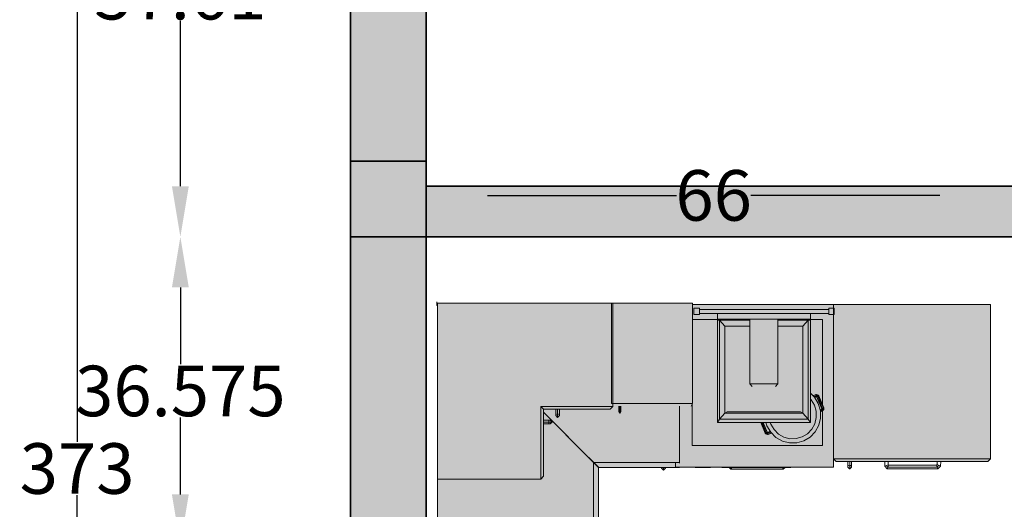
# Model space of a CAD drawing. Units: inches. Extents: x 1994 to 3075, y 3517 to 3950.
# Tile 50 of 58: x 2630 to 2747, y 3723 to 3781. Entities that reach past the tile are written whole.
import ezdxf

# ---------------------------------------------------------------- set-up
doc = ezdxf.new("R2010")
doc.units = ezdxf.units.IN
for name, color, linetype, lineweight in [('A-ANNO-DIMS', 2, 'Continuous', 18), ('A-COLS', 7, 'Continuous', 35), ('A-COLS-PATT', 6, 'Continuous', 13), ('A-FLOR-FIXT', 8, 'Continuous', 18), ('A-WALL', 7, 'Continuous', 35), ('A-WALL-PATT', 252, 'Continuous', 13)]:
    doc.layers.add(name, color=color, linetype=linetype, lineweight=lineweight)
doc.layers.add('hatch', color=254, linetype='Continuous')
doc.styles.get("Standard").update_dxf_attribs({"font": 'arial.ttf'})
doc.dimstyles.get("Standard").update_dxf_attribs({"dimtxt": 6, "dimasz": 6, "dimexe": 0.18, "dimexo": 0.0625, "dimgap": 0.09, "dimtad": 0, "dimtih": 1, "dimtoh": 1, "dimdec": 4, "dimzin": 0, "dimdsep": 46, "dimlunit": 4, "dimtxsty": 'Standard', "dimcen": 0.09, "dimse1": 1, "dimse2": 1, "dimadec": 0, "dimazin": 0, "dimtfac": 1, "dimtdec": 4, "dimtofl": 0, "dimtmove": 0, "dimatfit": 3, "dimfxl": 1, "dimtolj": 1, "dimtzin": 0, "dimarcsym": 0})

# ---------------------------------------------------------------- blocks, each defined once
blk = doc.blocks.new('kithen1')
at = {"layer": 'hatch'}
blk.add_hatch(color=256, dxfattribs=at).paths.add_polyline_path([(-2799.7, -8.3), (-2273.3, -8.3), (-2273.3, -1.7), (-2257.5, -1.7), (-2257.5, -1.1), (-1023.7, -1.1), (-1023.7, 0), (0, 0), (0, -0.3), (0.3, -0.3), (0.3, -1009.9), (-6.1, -1009.9), (-6.1, -2189.3), (-615.8, -2189.3), (-626.5, -2178.9), (-626.5, -1578.2), (-615.8, -1567.8), (-649.5, -1567.8), (-649.5, -1399.1), (-650.3, -1399.1), (-650.3, -1376.8), (-657.9, -1368.5), (-657.8, -1162.4), (-650.3, -1155.1), (-650.3, -1126.4), (-649.5, -1126.4), (-649.5, -1081.1), (-650.3, -1081.1), (-650.3, -1021.1), (-649.5, -1021.1), (-649.5, -959.1), (-651, -959.1), (-650.7, -903), (-653.5, -903), (-660.6, -895.5), (-660.5, -894.6), (-653.5, -887.1), (-651, -887.1), (-651, -638.7), (-651.2, -638.5), (-898.3, -638.5), (-898.3, -640.4), (-905.9, -647.4), (-906.8, -647.4), (-914.3, -640.4), (-914.3, -638.5), (-971.4, -638.5), (-971.4, -642.6), (-1016.2, -642.6), (-1016.2, -643.9), (-1023.8, -650.9), (-1024.7, -650.9), (-1032.2, -643.9), (-1032.2, -642.6), (-1179.7, -642.6), (-1188.8, -650.9), (-1395.6, -650.9), (-1403.7, -642.6), (-1813.5, -642.6), (-1822.6, -650.9), (-2029.4, -650.9), (-2037.5, -642.6), (-2257.5, -642.6), (-2257.5, -618.1), (-2261.3, -618.1), (-2271.7, -628.7), (-2458, -628.7), (-2727.7, -628.7), (-2727.7, -651.1), (-2735, -658.1), (-2735.9, -658), (-2743.2, -651.1), (-2743.2, -628.7), (-2789.4, -628.7), (-2799.7, -618.1)])
at = {"color": 0}
for p, q in [((0, 0), (-1023.7, 0)), ((-696.5, 0), (-696.5, -409.2)), ((-8.6, 1.9), (-10.5, 0)), ((-10.1, 0), (-8.2, 1.9)), ((-8.2, 1.9), (-8.3, 1.8)), ((-8.3, 1.9), (-8.3, 0)), ((5.4, 1.8), (-8.3, 1.8)), ((0, 0), (0, -694.7)), ((0, -0.3), (0, 0)), ((0.3, -0.3), (0, -0.3)), ((0.3, -671.1), (0.3, -0.3)), ((-696.5, -409.2), (-408.8, -409.2)), ((-685.5, -420.3), (-696.5, -409.2)), ((-419.9, -420.3), (-685.5, -420.3)), ((-432.1, -420.3), (-630.9, -618.1)), ((-630.6, -618.4), (-431.9, -420.3)), ((-614.8, -602.2), (-432.2, -420.3)), ((-431.9, -420.3), (-614.5, -602.5)), ((-432, -420.3), (-607.9, -595.8)), ((-432.1, -420.3), (-607.9, -595.4)), ((-478.5, -420.3), (-478.5, -439.9)), ((-470.7, -443), (-470.7, -420.3)), ((-462.9, -420.3), (-462.9, -439.9)), ((-408.8, -409.2), (-419.9, -420.3)), ((-419.9, -683.7), (-419.9, -420.3)), ((-408.8, -409.2), (-408.8, -694.7)), ((-478.5, -439.9), (-470.7, -443)), ((-478.5, -439.9), (-478.5, -446.8)), ((-478.5, -446.8), (-470.7, -454.1)), ((-462.9, -439.9), (-470.7, -443)), ((-470.7, -443), (-470.7, -454.1)), ((-470.7, -454.1), (-462.9, -446.8)), ((-462.9, -446.8), (-462.9, -439.9)), ((-444.9, -468.4), (-452.2, -476.2)), ((-452.2, -476.2), (-441.1, -476.2)), ((-452.2, -476.2), (-444.9, -484)), ((-419.9, -468.4), (-444.9, -468.4)), ((-444.9, -484), (-438, -484)), ((-441.1, -476.2), (-438, -468.4)), ((-419.9, -476.2), (-441.1, -476.2)), ((-441.1, -476.2), (-438, -484)), ((-438, -484), (-419.9, -484)), ((-540.1, -527.9), (-540.1, -528.1)), ((-597, -584.5), (-597, -584.9)), ((-630.9, -618.1), (-971.4, -618.1)), ((-611.6, -599.1), (-651.2, -638.5)), ((-611.6, -599.4), (-651, -638.7)), ((-642.6, -629.8), (-630.9, -618.1)), ((-630.6, -618.4), (-642.3, -630.1)), ((-630.9, -618.1), (-614.8, -602.2)), ((-614.5, -602.5), (-630.6, -618.4)), ((-630.6, -959.1), (-630.6, -618.4)), ((-620.1, -607.7), (-609.4, -597.1)), ((-619.9, -607.6), (-620.1, -607.6)), ((-620.1, -607.9), (-620.1, -607.7)), ((-609, -596.9), (-609.4, -596.9)), ((-609.4, -597.1), (-609.4, -597.2)), ((-607.9, -595.4), (-607.9, -595.8)), ((-651.2, -638.5), (-971.4, -638.5)), ((-651, -638.7), (-651, -959.1)), ((-408.8, -694.7), (-419.9, -683.7)), ((0, -694.7), (-408.8, -694.7)), ((-0.1, -689.2), (-397.2, -689.2)), ((-397.2, -689.2), (-397.2, -1009.9)), ((-0.1, -1009.9), (-0.1, -689.2)), ((-0.1, -699.8), (-0.1, -998.7)), ((0.3, -700.4), (-0.1, -700.4)), ((0, -694.7), (0, -671.1)), ((0, -671.1), (0.3, -671.1)), ((0.3, -998.7), (0.3, -700.4)), ((-429, -718.2), (-436, -721.9)), ((-436, -721.9), (-425.3, -721.9)), ((-436, -721.9), (-429, -725.7)), ((-407.9, -718.2), (-429, -718.2)), ((-429, -725.7), (-422.2, -725.7)), ((-425.3, -721.9), (-422.2, -718.2)), ((-407.9, -721.9), (-425.3, -721.9)), ((-425.3, -721.9), (-422.2, -725.7)), ((-422.2, -725.7), (-407.9, -725.7)), ((-653.5, -887.9), (-660.6, -895.5)), ((-660.6, -895.5), (-660.5, -894.6)), ((-660.6, -895.5), (-651, -895.5)), ((-653.5, -903), (-660.6, -895.5)), ((-660.5, -894.6), (-653.5, -887.1)), ((-651, -887), (-653.5, -887.1)), ((-653.5, -887.1), (-652.7, -887.9)), ((-653.5, -887.1), (-653.5, -887.9)), ((-653.5, -887.9), (-651, -887.9)), ((-651, -903), (-653.5, -903)), ((-651, -959.1), (-649.5, -959.1)), ((-633.4, -942.7), (-649.5, -942.7)), ((-649.5, -942.7), (-649.5, -1567.8)), ((-630.6, -959.1), (-633.4, -959.1)), ((-407.9, -959.1), (-630.6, -959.1)), ((-398.5, -1009.2), (-564.1, -1009.2)), ((-564.1, -1009.2), (-564.1, -1525)), ((-397.2, -1009.9), (-407.9, -1004.5)), ((-397.2, -1009.9), (-0.1, -1009.9)), ((-65.6, -1009.9), (-65.6, -1108.4)), ((-6.1, -1009.9), (-6.1, -1567.8)), ((-0.1, -998.7), (0.3, -998.7)), ((-649.5, -1021.1), (-650.3, -1021.1)), ((-650.3, -1021.1), (-650.3, -1081.1)), ((-20.3, -1015.5), (-44.8, -1015.5)), ((-44.8, -1015.5), (-44.8, -1037.5)), ((-44.8, -1037.5), (-20.3, -1037.5)), ((-24.8, -1038), (-40.6, -1038)), ((-40.6, -1038), (-40.6, -1549.4)), ((-24.8, -1549.4), (-24.8, -1038)), ((-20.3, -1037.5), (-20.3, -1015.5)), ((-650.3, -1081.1), (-649.5, -1081.1)), ((-649.5, -1126.4), (-650.3, -1126.4)), ((-650.3, -1126.4), (-650.3, -1186.4)), ((-62.5, -1108.4), (-473.1, -1108.4)), ((-473.1, -1108.4), (-459.2, -1117.2)), ((-473.1, -1108.4), (-473.1, -1476.7)), ((-459.2, -1117.2), (-68.2, -1117.2)), ((-459.2, -1467.9), (-459.2, -1117.2)), ((-459.2, -1117.2), (-435.9, -1138.2)), ((-91.6, -1138.2), (-68.2, -1117.2)), ((-68.2, -1117.2), (-67.2, -1115.5)), ((-68.2, -1117.2), (-68.2, -1237.1)), ((-64.1, -1108.4), (-67.2, -1111.2)), ((-67.2, -1111.2), (-67.2, -1237.1)), ((-40.9, -1108.4), (-64.1, -1108.4)), ((-64.1, -1108.4), (-64.1, -1476.7)), ((-40.9, -1476.7), (-40.9, -1108.4)), ((-657.8, -1162.4), (-657.9, -1368.5)), ((-650.3, -1155.1), (-657.8, -1162.4)), ((-657.8, -1162.4), (-650.8, -1165.4)), ((-650.8, -1165.4), (-650.3, -1164.8)), ((-650.8, -1365.8), (-650.8, -1165.4)), ((-650.8, -1165.4), (-650.3, -1165.6)), ((-435.9, -1138.2), (-91.6, -1138.2)), ((-435.9, -1138.2), (-430.1, -1147)), ((-435.9, -1447), (-435.9, -1138.2)), ((-430.1, -1147), (-430.1, -1438.2)), ((-91.6, -1138.2), (-91.6, -1237.1)), ((-650.3, -1186.4), (-649.5, -1186.4)), ((-649.5, -1231.7), (-650.3, -1231.7)), ((-650.3, -1231.7), (-650.3, -1291.7)), ((-320.2, -1237.1), (-330.5, -1246.3)), ((-64.3, -1237.1), (-320.2, -1237.1)), ((-320.2, -1237.1), (-320.2, -1348.4)), ((-64.3, -1348.4), (-64.3, -1237.1)), ((-473.1, -1280.2), (-515, -1298.2)), ((-473.1, -1282.1), (-514, -1299.7)), ((-473.1, -1286.3), (-512, -1302.3)), ((-650.3, -1291.7), (-649.5, -1291.7)), ((-511.4, -1319.5), (-531.9, -1340.4)), ((-519.1, -1303.5), (-520.1, -1306.8)), ((-520.1, -1306.8), (-520.1, -1310.2)), ((-520.1, -1310.2), (-514.9, -1323)), ((-517.4, -1300.6), (-519.1, -1303.5)), ((-517.7, -1304.5), (-518.6, -1307.4)), ((-518.6, -1307.4), (-518.6, -1310.5)), ((-518.6, -1310.5), (-513.9, -1322)), ((-516.2, -1301.9), (-517.7, -1304.5)), ((-515.4, -1308), (-517.7, -1304.5)), ((-515, -1298.2), (-517.4, -1300.6)), ((-514, -1299.7), (-516.2, -1301.9)), ((-515.4, -1308), (-516.2, -1301.9)), ((-514, -1299.7), (-515.4, -1308)), ((-512, -1302.3), (-515.4, -1308)), ((-515.4, -1308), (-512.4, -1308.2)), ((-511.2, -1319.3), (-515.4, -1308)), ((-512, -1302.3), (-514, -1299.7)), ((-511.2, -1305.5), (-512.4, -1308.2)), ((-512.4, -1308.2), (-511.3, -1307.8)), ((-512.4, -1308.2), (-508, -1317.5)), ((-512.4, -1308.2), (-508.5, -1317.7)), ((-508.7, -1317.8), (-512.4, -1308.2)), ((-511.2, -1305.5), (-512, -1302.3)), ((-486.2, -1304.5), (-511.4, -1319.5)), ((-511.3, -1307.8), (-510.4, -1305.8)), ((-511.3, -1307.8), (-507.6, -1317.2)), ((-473.1, -1289.8), (-511.2, -1305.5)), ((-510.4, -1305.8), (-511.2, -1305.5)), ((-473.1, -1290.3), (-510.4, -1305.8)), ((-479.5, -1319.9), (-500.9, -1332.7)), ((-473.1, -1300.7), (-486.2, -1304.5)), ((-473.1, -1318.1), (-479.5, -1319.9)), ((-649.5, -1339.1), (-650.3, -1339.1)), ((-650.3, -1339.1), (-650.3, -1399.1)), ((-531.9, -1340.4), (-546.3, -1365.8)), ((-518.2, -1350.4), (-530.4, -1372)), ((-500.9, -1332.7), (-518.2, -1350.4)), ((-320.2, -1348.4), (-330.5, -1339.2)), ((-320.2, -1348.4), (-64.3, -1348.4)), ((-91.6, -1447), (-91.6, -1348.4)), ((-68.2, -1348.4), (-68.2, -1467.9)), ((-67.2, -1474), (-67.2, -1348.4)), ((-657.9, -1368.5), (-650.8, -1365.8)), ((-657.9, -1368.5), (-650.3, -1376.8)), ((-650.3, -1365.6), (-650.8, -1365.8)), ((-650.8, -1365.8), (-650.3, -1366.5)), ((-650.3, -1399.1), (-649.5, -1399.1)), ((-546.3, -1365.8), (-553.5, -1394)), ((-553.5, -1394), (-553.2, -1423)), ((-530.4, -1372), (-536.6, -1395.8)), ((-536.6, -1395.8), (-536.3, -1420.4)), ((-553.2, -1423), (-545.3, -1450.9)), ((-536.3, -1420.4), (-529.6, -1444.1)), ((-430.1, -1438.2), (-435.9, -1447)), ((-545.3, -1450.9), (-530.3, -1475.7)), ((-530.3, -1475.7), (-509.3, -1495.8)), ((-529.6, -1444.1), (-516.9, -1465.1)), ((-516.9, -1465.1), (-499.1, -1482.2)), ((-473.1, -1476.7), (-459.2, -1467.9)), ((-162.2, -1476.7), (-473.1, -1476.7)), ((-473.1, -1476.7), (-64.1, -1476.7)), ((-435.9, -1447), (-459.2, -1467.9)), ((-459.2, -1467.9), (-68.2, -1467.9)), ((-91.6, -1447), (-435.9, -1447)), ((-404.5, -1492.5), (-383.1, -1479.8)), ((-383.1, -1479.8), (-380.1, -1476.7)), ((-372.5, -1493), (-356.6, -1476.7)), ((-68.2, -1467.9), (-91.6, -1447)), ((-68.2, -1467.9), (-67.2, -1469.6)), ((-64.1, -1476.7), (-67.2, -1474)), ((-65.6, -1476.7), (-65.6, -1525)), ((-64.1, -1476.7), (-40.9, -1476.7)), ((-509.3, -1495.8), (-483.7, -1509.8)), ((-499.1, -1482.2), (-477.4, -1494)), ((-483.7, -1509.8), (-455.3, -1516.7)), ((-477.4, -1494), (-453.3, -1499.9)), ((-455.3, -1516.7), (-426, -1516.1)), ((-453.3, -1499.9), (-428.4, -1499.4)), ((-426.6, -1525.5), (-430.8, -1516.2)), ((-429.6, -1516.2), (-425.8, -1524.2)), ((-428.4, -1499.4), (-404.5, -1492.5)), ((-423.4, -1522.1), (-426.1, -1516.1)), ((-426, -1516.1), (-397.7, -1508)), ((-420.8, -1520.4), (-423.3, -1515.3)), ((-422.4, -1515.1), (-419.6, -1520.1)), ((-419.6, -1520.1), (-421.9, -1514.9)), ((-419.6, -1520.1), (-420.8, -1520.4)), ((-417.9, -1521.4), (-419.6, -1520.1)), ((-371, -1502.5), (-418.6, -1522)), ((-371.9, -1502.2), (-417.9, -1521.4)), ((-417.7, -1525.2), (-370.2, -1505.7)), ((-368.3, -1508.3), (-414.8, -1528.3)), ((-367.2, -1509.7), (-414.4, -1530.1)), ((-397.7, -1508), (-372.5, -1493)), ((-371, -1500.1), (-373.6, -1493.6)), ((-373, -1493.3), (-369.9, -1499.8)), ((-369.9, -1499.8), (-372.7, -1493.1)), ((-372.5, -1493), (-369.9, -1499.8)), ((-371, -1500.1), (-371.9, -1502.2)), ((-371.9, -1502.2), (-371, -1502.5)), ((-371, -1502.5), (-369.9, -1499.8)), ((-369.9, -1499.8), (-371, -1500.1)), ((-370.2, -1505.7), (-371, -1502.5)), ((-366.9, -1500), (-370.3, -1490.7)), ((-366.9, -1500), (-370.2, -1505.7)), ((-370.2, -1505.7), (-368.3, -1508.3)), ((-369.9, -1499.8), (-366.9, -1500)), ((-368.3, -1508.3), (-366.9, -1500)), ((-366.1, -1506.1), (-368.3, -1508.3)), ((-367.6, -1488), (-363.7, -1497.5)), ((-364.8, -1507.3), (-367.2, -1509.7)), ((-364.5, -1503.5), (-366.9, -1500)), ((-366.9, -1500), (-366.1, -1506.1)), ((-366.6, -1486.9), (-362.2, -1497.8)), ((-366.1, -1506.1), (-364.5, -1503.5)), ((-363.1, -1504.4), (-364.8, -1507.3)), ((-363.7, -1500.6), (-364.5, -1503.5)), ((-363.7, -1497.5), (-363.7, -1500.6)), ((-362.2, -1501.2), (-363.1, -1504.4)), ((-362.2, -1497.8), (-362.2, -1501.2)), ((-564.1, -1525), (-426.8, -1525)), ((-424.2, -1527.8), (-426.6, -1525.5)), ((-425.8, -1524.2), (-423.6, -1526.3)), ((-421.2, -1529.4), (-424.2, -1527.8)), ((-423.6, -1526.3), (-423.4, -1522.1)), ((-420.9, -1527.8), (-423.6, -1526.3)), ((-420.8, -1520.4), (-423.4, -1522.1)), ((-423.4, -1522.1), (-417.7, -1525.2)), ((-417.9, -1530.2), (-421.2, -1529.4)), ((-417.7, -1525.2), (-420.9, -1527.8)), ((-420.9, -1527.8), (-418, -1528.4)), ((-418.6, -1522), (-420.8, -1520.4)), ((-418.6, -1522), (-417.9, -1521.4)), ((-417.7, -1525.2), (-418.6, -1522)), ((-418, -1528.4), (-414.8, -1528.3)), ((-414.4, -1530.1), (-417.9, -1530.2)), ((-414.8, -1528.3), (-417.7, -1525.2)), ((-65.6, -1525), (-402.7, -1525)), ((-20.3, -1549.4), (-44.8, -1549.4)), ((-44.8, -1549.4), (-44.8, -1571.3)), ((-20.3, -1571.3), (-20.3, -1549.4)), ((-44.8, -1567.8), (-649.5, -1567.8)), ((-626.5, -1578.2), (-615.8, -1567.8)), ((-626.5, -2178.9), (-626.5, -1578.2)), ((-6.1, -1567.8), (-615.8, -1567.8)), ((-615.8, -1567.8), (-615.8, -2189.3)), ((-44.8, -1571.3), (-20.3, -1571.3)), ((-6.1, -1567.8), (-20.3, -1567.8)), ((-6.1, -2189.3), (-6.1, -1567.8)), ((-655.9, -1632.5), (-648.9, -1625.2)), ((-655.8, -1631.6), (-655.9, -1632.5)), ((-645.2, -1632.6), (-655.9, -1632.5)), ((-655.9, -1632.5), (-648.9, -1639.8)), ((-648.9, -1624.4), (-655.8, -1631.6)), ((-648.9, -1624.4), (-642.6, -1624.3)), ((-648.9, -1625.2), (-648.9, -1624.4)), ((-648.1, -1625.2), (-648.9, -1624.4)), ((-642.1, -1625.2), (-648.9, -1625.2)), ((-642.1, -1625.2), (-645.2, -1632.6)), ((-642.1, -1639.8), (-645.2, -1632.6)), ((-645.2, -1632.6), (-626.5, -1632.6)), ((-626.5, -1624.3), (-642.6, -1624.3)), ((-642.6, -1624.3), (-642.3, -1625.2)), ((-626.5, -1625.2), (-642.1, -1625.2)), ((-648.9, -1639.8), (-642.1, -1639.8)), ((-626.5, -1639.8), (-642.1, -1639.8)), ((-655.8, -1781), (-655.9, -1980.9)), ((-655.8, -1781), (-645.4, -1771.2)), ((-648.9, -1783.9), (-655.8, -1781)), ((-648.9, -1783.9), (-642.6, -1777.9)), ((-641.9, -1786.7), (-648.9, -1783.9)), ((-648.9, -1978.3), (-648.9, -1783.9)), ((-626.5, -1770.8), (-645.4, -1771.2)), ((-645.4, -1771.2), (-639.8, -1784.7)), ((-639.8, -1784.7), (-641.9, -1786.7)), ((-641.9, -1786.7), (-641.8, -1975.6)), ((-626.5, -1785), (-639.8, -1784.7)), ((-655.9, -1980.9), (-648.9, -1978.3)), ((-645.2, -1992.2), (-655.9, -1980.9)), ((-641.8, -1975.6), (-648.9, -1978.3)), ((-648.9, -1978.3), (-642.1, -1985.5)), ((-645.2, -1992.2), (-639.1, -1978.9)), ((-641.8, -1975.6), (-639.1, -1978.9)), ((-639.1, -1978.9), (-626.5, -1978.6)), ((-626.5, -1992.6), (-645.2, -1992.2)), ((-626.5, -2178.9), (-615.8, -2189.3)), ((-615.8, -2189.3), (-6.1, -2189.3))]:
    blk.add_line(p, q, dxfattribs=at)
blk.add_lwpolyline([(-1023.7, 0), (0, 0), (0, -0.3), (0.3, -0.3), (0.3, -1009.9), (-6.1, -1009.9), (-6.1, -2189.3), (-615.8, -2189.3), (-626.5, -2178.9), (-626.5, -1578.2), (-615.8, -1567.8), (-649.5, -1567.8), (-649.5, -1399.1), (-650.3, -1399.1), (-650.3, -1376.8), (-657.9, -1368.5), (-657.8, -1162.4), (-650.3, -1155.1), (-650.3, -1126.4), (-649.5, -1126.4), (-649.5, -1081.1), (-650.3, -1081.1), (-650.3, -1021.1), (-649.5, -1021.1), (-649.5, -959.1), (-651, -959.1), (-650.7, -903), (-653.5, -903), (-660.6, -895.5), (-660.5, -894.6), (-653.5, -887.1), (-651, -887.1), (-651, -638.7), (-651.2, -638.5), (-898.3, -638.5)])
blk = doc.blocks.new('*D29')
at = {"layer": 'A-ANNO-DIMS', "color": 0, "lineweight": -2, "transparency": 16777216}
for p, q in [((2757.66, 3741.43), (2757.66, 3708.56)), ((2757.66, 3669.3), (2757.66, 3702.17))]:
    blk.add_line(p, q, dxfattribs=at)
at = {"layer": 'A-ANNO-DIMS', "color": 0, "transparency": 16777216}
for points in [[(2756.66, 3741.43), (2758.66, 3741.43), (2757.66, 3747.43)], [(2756.66, 3669.3), (2758.66, 3669.3), (2757.66, 3663.3)]]:
    blk.add_solid(points, dxfattribs=at)
at = {"layer": 'Defpoints', "color": 0, "transparency": 16777216}
for p in [(2745.04, 3747.43), (2757.66, 3747.43), (2745.04, 3663.3)]:
    blk.add_point(p, dxfattribs=at)
at = {"layer": 'A-ANNO-DIMS', "color": 0, "transparency": 16777216, "insert": (2757.66, 3705.36), "char_height": 6, "attachment_point": 5}
blk.add_mtext('\\A1;KITCHEN UNIT 84', dxfattribs=at)
blk = doc.blocks.new('*D30')
at = {"layer": 'A-ANNO-DIMS', "color": 0, "lineweight": -2, "transparency": 16777216}
for p, q in [((2685.33, 3760.05), (2707.78, 3760.05)), ((2739.04, 3760.05), (2716.59, 3760.05))]:
    blk.add_line(p, q, dxfattribs=at)
at = {"layer": 'A-ANNO-DIMS', "color": 0, "transparency": 16777216}
for points in [[(2685.33, 3761.05), (2685.33, 3759.05), (2679.33, 3760.05)], [(2739.04, 3761.05), (2739.04, 3759.05), (2745.04, 3760.05)]]:
    blk.add_solid(points, dxfattribs=at)
at = {"layer": 'Defpoints', "color": 0, "transparency": 16777216}
for p in [(2679.33, 3760.05), (2679.33, 3747.43), (2745.04, 3747.43)]:
    blk.add_point(p, dxfattribs=at)
at = {"layer": 'A-ANNO-DIMS', "color": 0, "transparency": 16777216, "insert": (2712.19, 3760.05), "char_height": 6, "attachment_point": 5}
blk.add_mtext('\\A1;66', dxfattribs=at)
blk = doc.blocks.new('*D32')
at = {"layer": 'A-ANNO-DIMS', "color": 0, "lineweight": -2, "transparency": 16777216}
for p, q in [((2636.61, 3908.13), (2636.61, 3730.78)), ((2636.61, 3547.13), (2636.61, 3724.47))]:
    blk.add_line(p, q, dxfattribs=at)
at = {"layer": 'A-ANNO-DIMS', "color": 0, "transparency": 16777216}
for points in [[(2635.61, 3908.13), (2637.61, 3908.13), (2636.61, 3914.13)], [(2635.61, 3547.13), (2637.61, 3547.13), (2636.61, 3541.13)]]:
    blk.add_solid(points, dxfattribs=at)
at = {"layer": 'Defpoints', "color": 0, "transparency": 16777216}
for p in [(2636.61, 3914.13), (2669.07, 3914.13), (2810.07, 3541.13)]:
    blk.add_point(p, dxfattribs=at)
at = {"layer": 'A-ANNO-DIMS', "color": 0, "transparency": 16777216, "insert": (2636.61, 3727.63), "char_height": 6, "attachment_point": 5}
blk.add_mtext('\\A1;373', dxfattribs=at)
blk = doc.blocks.new('*D44')
at = {"layer": 'A-ANNO-DIMS', "color": 0, "lineweight": -2, "transparency": 16777216}
for p, q in [((2648.87, 3806.74), (2648.87, 3787.09)), ((2648.87, 3761.13), (2648.87, 3780.78))]:
    blk.add_line(p, q, dxfattribs=at)
at = {"layer": 'A-ANNO-DIMS', "color": 0, "transparency": 16777216}
for points in [[(2647.87, 3806.74), (2649.87, 3806.74), (2648.87, 3812.74)], [(2647.87, 3761.13), (2649.87, 3761.13), (2648.87, 3755.13)]]:
    blk.add_solid(points, dxfattribs=at)
at = {"layer": 'Defpoints', "color": 0, "transparency": 16777216}
for p in [(2648.87, 3812.74), (2669.07, 3812.74), (2669.07, 3755.13)]:
    blk.add_point(p, dxfattribs=at)
at = {"layer": 'A-ANNO-DIMS', "color": 0, "transparency": 16777216, "insert": (2648.87, 3783.93), "char_height": 6, "attachment_point": 5}
blk.add_mtext('\\A1;57.61', dxfattribs=at)
blk = doc.blocks.new('*D46')
at = {"layer": 'A-ANNO-DIMS', "color": 0, "lineweight": -2, "transparency": 16777216}
for p, q in [((2648.87, 3749.13), (2648.87, 3740)), ((2648.87, 3724.55), (2648.87, 3733.68))]:
    blk.add_line(p, q, dxfattribs=at)
at = {"layer": 'A-ANNO-DIMS', "color": 0, "transparency": 16777216}
for points in [[(2647.87, 3749.13), (2649.87, 3749.13), (2648.87, 3755.13)], [(2647.87, 3724.55), (2649.87, 3724.55), (2648.87, 3718.55)]]:
    blk.add_solid(points, dxfattribs=at)
at = {"layer": 'Defpoints', "color": 0, "transparency": 16777216}
for p in [(2648.87, 3755.13), (2669.07, 3755.13), (2669.07, 3718.55)]:
    blk.add_point(p, dxfattribs=at)
at = {"layer": 'A-ANNO-DIMS', "color": 0, "transparency": 16777216, "insert": (2648.87, 3736.84), "char_height": 6, "attachment_point": 5}
blk.add_mtext('\\A1;36.575', dxfattribs=at)

msp = doc.modelspace()

# ---------------------------------------------------------------- hatches: boundary and pattern name
at = {"layer": 'A-COLS-PATT'}
h = msp.add_hatch(color=256, dxfattribs=at)
h.dxf.hatch_style = 1
h.paths.add_polyline_path([(2678.072, 3914.1269), (2669.072, 3914.1269), (2669.072, 3905.1269), (2678.072, 3905.1269)])
h.paths.add_polyline_path([(2816.072, 3914.1269), (2807.072, 3914.1269), (2807.072, 3905.1269), (2816.072, 3905.1269)])
h.paths.add_polyline_path([(2894.9096, 3914.1269), (2885.9096, 3914.1269), (2885.9096, 3905.1269), (2894.9096, 3905.1269)])
h.paths.add_polyline_path([(3033.072, 3914.1269), (3024.072, 3914.1269), (3024.072, 3905.1269), (3033.072, 3905.1269)])
h.paths.add_polyline_path([(3033.072, 3764.1269), (3024.072, 3764.1269), (3024.072, 3755.1269), (3033.072, 3755.1269)])
h.paths.add_polyline_path([(2895.072, 3764.1269), (2886.072, 3764.1269), (2886.072, 3755.1269), (2895.072, 3755.1269)])
h.paths.add_polyline_path([(2816.072, 3764.1269), (2807.072, 3764.1269), (2807.072, 3755.1269), (2816.072, 3755.1269)])
h.paths.add_polyline_path([(2678.072, 3764.1269), (2669.072, 3764.1269), (2669.072, 3755.1269), (2678.072, 3755.1269)])
h.paths.add_polyline_path([(2678.072, 3664.1269), (2669.072, 3664.1269), (2669.072, 3655.1269), (2678.072, 3655.1269)])
h.paths.add_polyline_path([(2816.072, 3664.1269), (2807.072, 3664.1269), (2807.072, 3655.1269), (2816.072, 3655.1269)])
h.paths.add_polyline_path([(3033.072, 3616.1269), (3024.072, 3616.1269), (3024.072, 3607.1269), (3033.072, 3607.1269)])
h.paths.add_polyline_path([(2894.9096, 3616.1269), (2885.9096, 3616.1269), (2885.9096, 3607.1269), (2894.9096, 3607.1269)])
h.paths.add_polyline_path([(2816.072, 3559.1269), (2807.072, 3559.1269), (2807.072, 3550.1269), (2816.072, 3550.1269)])
h.paths.add_polyline_path([(2678.072, 3559.1269), (2669.072, 3559.1269), (2669.072, 3550.1269), (2678.072, 3550.1269)])
at = {"layer": 'A-WALL-PATT'}
h = msp.add_hatch(color=256, dxfattribs=at)
h.dxf.hatch_style = 1
h.paths.add_polyline_path([(2678.072, 3755.1269), (2669.072, 3755.1269), (2669.072, 3718.5523), (2678.072, 3718.5523)])
h.paths.add_polyline_path([(2807.072, 3761.1269), (2678.072, 3761.1269), (2678.072, 3755.1269), (2807.072, 3755.1269)])
h.paths.add_polyline_path([(2678.072, 3812.7371), (2669.072, 3812.7371), (2669.072, 3809.7371), (2669.072, 3764.1269), (2678.072, 3764.1269)])
h.paths.add_polyline_path([(2678.072, 3905.1269), (2669.072, 3905.1269), (2669.072, 3868.7491), (2678.072, 3868.7491)])
h.paths.add_polyline_path([(2723.826, 3914.1269), (2720.826, 3914.1269), (2678.072, 3914.1269), (2678.072, 3905.1269), (2723.826, 3905.1269)])
h.paths.add_polyline_path([(2807.072, 3914.1269), (2779.838, 3914.1269), (2779.838, 3905.1269), (2807.072, 3905.1269)])
h.paths.add_polyline_path([(2837.6979, 3914.1269), (2834.6979, 3914.1269), (2820.9062, 3914.1269), (2816.072, 3914.1269), (2816.072, 3905.1269), (2837.6979, 3905.1269)])
h.paths.add_polyline_path([(2885.9096, 3914.1269), (2869.71, 3914.1269), (2869.71, 3905.1269), (2876.9183, 3905.1269), (2885.9096, 3905.1269)])
h.paths.add_polyline_path([(2933.6904, 3914.1269), (2930.6904, 3914.1269), (2894.9096, 3914.1269), (2894.9096, 3905.1269), (2933.6904, 3905.1269)])
h.paths.add_polyline_path([(3024.072, 3914.1269), (2989.7025, 3914.1269), (2989.7025, 3905.1269), (3024.072, 3905.1269)])
h.paths.add_polyline_path([(3033.072, 3905.1269), (3024.072, 3905.1269), (3024.072, 3861.4192), (3033.072, 3861.4192)])
h.paths.add_polyline_path([(3033.072, 3805.4072), (3024.072, 3805.4072), (3024.072, 3764.1269), (3033.072, 3764.1269)])
h.paths.add_polyline_path([(3033.072, 3755.1269), (3024.072, 3755.1269), (3024.072, 3732.1247), (3033.072, 3732.1247), (3033.072, 3735.1247)])
h.paths.add_polyline_path([(3024.072, 3761.1269), (2895.072, 3761.1269), (2895.072, 3755.1269), (3024.072, 3755.1269)])
h.paths.add_polyline_path([(3033.072, 3676.1126), (3024.072, 3676.1126), (3024.072, 3616.1269), (3033.072, 3616.1269)])
h.paths.add_polyline_path([(3024.072, 3613.1269), (2959.4908, 3613.1269), (2959.4908, 3607.1269), (3024.072, 3607.1269)])
h.paths.add_polyline_path([(2914.1254, 3613.1269), (2894.9096, 3613.1269), (2894.9096, 3607.1269), (2914.1254, 3607.1269)])
h.paths.add_polyline_path([(2885.9096, 3613.1269), (2852.072, 3613.1269), (2852.072, 3607.1269), (2885.9096, 3607.1269)])
h.paths.add_polyline_path([(2822.072, 3613.1269), (2810.072, 3613.1269), (2810.072, 3559.1269), (2816.072, 3559.1269), (2816.072, 3607.1269), (2822.072, 3607.1269)])
h.paths.add_polyline_path([(2933.072, 3607.1269), (2924.072, 3607.1269), (2924.072, 3550.1269), (2892.072, 3550.1269), (2816.072, 3550.1269), (2810.072, 3550.1269), (2810.072, 3541.1269), (2892.072, 3541.1269), (2933.072, 3541.1269)])
h.paths.add_polyline_path([(2807.072, 3559.1269), (2678.072, 3559.1269), (2678.072, 3550.1269), (2807.072, 3550.1269)])
h.paths.add_polyline_path([(2678.072, 3655.1269), (2669.072, 3655.1269), (2669.072, 3559.1269), (2678.072, 3559.1269)])
h.paths.add_polyline_path([(2678.072, 3686.5403), (2669.072, 3686.5403), (2669.072, 3664.1269), (2678.072, 3664.1269)])
h.paths.add_polyline_path([(2807.072, 3661.1269), (2678.072, 3661.1269), (2678.072, 3655.1269), (2807.072, 3655.1269)])
h.paths.add_polyline_path([(2816.072, 3755.1269), (2810.072, 3755.1269), (2810.072, 3703.1269), (2816.072, 3703.1269)])
h.paths.add_polyline_path([(2816.072, 3905.1269), (2810.072, 3905.1269), (2810.072, 3803.1269), (2816.072, 3803.1269), (2816.072, 3815.1269)])
h.paths.add_polyline_path([(2886.072, 3821.1269), (2852.072, 3821.1269), (2852.072, 3815.1269), (2886.072, 3815.1269)])
h.paths.add_polyline_path([(2822.072, 3821.1269), (2816.072, 3821.1269), (2816.072, 3815.1269), (2822.072, 3815.1269)])
h.paths.add_polyline_path([(2892.072, 3905.1269), (2886.072, 3905.1269), (2886.072, 3803.1269), (2892.072, 3803.1269)])

# ---------------------------------------------------------------- linework, layer by layer
at = {"layer": 'A-COLS'}
msp.add_lwpolyline([(2669.072, 3755.1269), (2678.072, 3755.1269), (2678.072, 3764.1269), (2669.072, 3764.1269)], close=True, dxfattribs=at)
at = {"layer": 'A-WALL'}
for p, q in [((2669.072, 3914.1269), (2669.072, 3550.1269)), ((2678.072, 3905.1269), (2678.072, 3761.1269)), ((2678.072, 3761.1269), (2807.072, 3761.1269)), ((2678.072, 3755.1269), (2810.072, 3755.1269)), ((2678.072, 3755.1269), (2678.072, 3661.1269))]:
    msp.add_line(p, q, dxfattribs=at)

# ---------------------------------------------------------------- block references
at = {"layer": 'A-FLOR-FIXT', "xscale": 0.0299911025630211, "yscale": 0.0299911025630211, "zscale": 0.0299911025630211, "rotation": 89.99999999999999}
msp.add_blockref('kithen1', (2679.3854, 3747.2678), dxfattribs=at)

# ---------------------------------------------------------------- dimensions: what is measured, and where the dimension line sits
at = {"layer": 'A-ANNO-DIMS'}
for base, p1, p2, angle, override, picture, middle in [((2636.6096, 3914.1269), (2810.072, 3541.1269), (2669.072, 3914.1269), 90, {"dimdec": 0, "dimlfac": 1, "dimrnd": 0, "dimzin": 0, "dimdsep": 46, "dimlunit": 2}, '*D32', (2636.6096, 3727.6269)), ((2648.872, 3812.7371), (2669.072, 3755.1269), (2669.072, 3812.7371), 90, {"dimdec": 2, "dimlfac": 1, "dimrnd": 0, "dimzin": 0, "dimdsep": 46, "dimlunit": 2}, '*D44', (2648.872, 3783.932)), ((2679.3281, 3760.0476), (2745.0442, 3747.4285), (2679.3281, 3747.4285), 180, {"dimdec": 0, "dimlfac": 1, "dimrnd": 0, "dimzin": 0, "dimdsep": 46, "dimlunit": 2}, '*D30', (2712.1862, 3760.0476)), ((2648.872, 3755.1269), (2669.072, 3718.5523), (2669.072, 3755.1269), 90, {"dimdec": 3, "dimlfac": 1, "dimrnd": 0, "dimzin": 0, "dimdsep": 46, "dimlunit": 2}, '*D46', (2648.872, 3736.8396))]:
    dim = msp.add_linear_dim(base=base, p1=p1, p2=p2, angle=angle, dimstyle='Standard', override=override, dxfattribs=at)
    dim.commit()
    dim.dimension.update_dxf_attribs({"geometry": picture, "text_midpoint": middle})
dim = msp.add_linear_dim(base=(2757.6633, 3747.4285), p1=(2745.0442, 3663.3012), p2=(2745.0442, 3747.4285), angle=90, text='KITCHEN UNIT <>', dimstyle='Standard', override={"dimdec": 0, "dimlfac": 1, "dimrnd": 0, "dimzin": 0, "dimdsep": 46, "dimlunit": 2}, dxfattribs=at)
dim.commit()
dim.dimension.update_dxf_attribs({"geometry": '*D29', "text_midpoint": (2757.6633, 3705.3649)})

doc.saveas('drawing.dxf')
